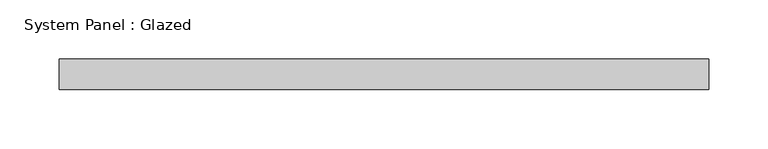
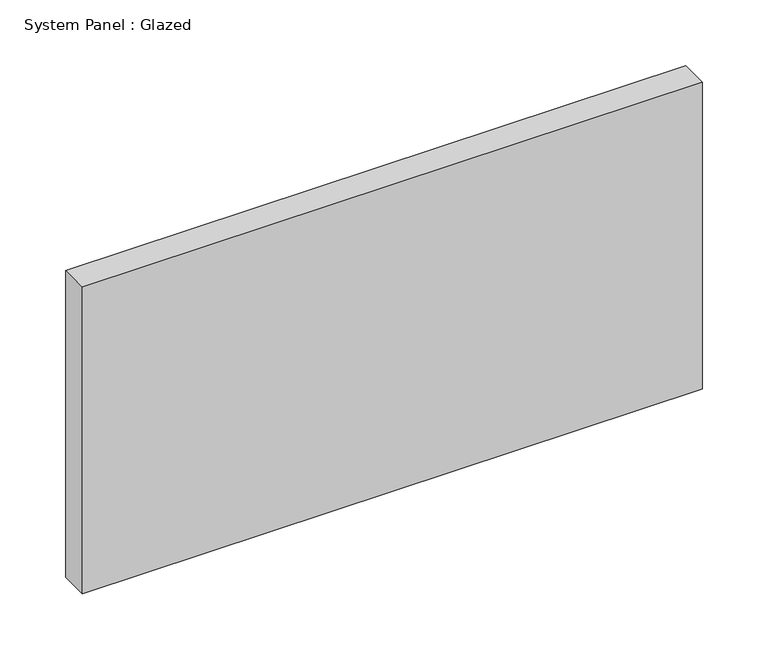
"""IFC4 building model written with IfcOpenShell, lengths in millimetres: plate geometry, System Panel : Glazed."""

from ifc_helpers import new_model, si_unit, origin, origin_with_axes, place, context, project, spatial, polyline, outline, extrude, source, transform, mapped, element, save


def system_panel_glazed_c61bacb6(model_context):
    return source(origin(), model_context, "Body", "SweptSolid", [
        extrude(outline(polyline([(273.05, 19.05), (-273.05, 19.05), (-273.05, 44.45), (273.05, 44.45), (273.05, 19.05)])), origin_with_axes(), (0.0, 0.0, 1.0), 285.75),
    ])


if __name__ == "__main__":
    model = new_model("IFC4")
    model_context = context("Model", 3, world=origin())
    ifc_project = project(units=[si_unit("LENGTHUNIT", "METRE", prefix="MILLI")], contexts=[model_context])
    site = spatial("IfcSite", under=ifc_project)
    building = spatial("IfcBuilding", under=site)
    placement = place(None, origin())
    system_panel_glazed_shape = system_panel_glazed_c61bacb6(model_context)
    element("IfcPlate", 1, ObjectType="System Panel : Glazed", at=placement, inside=building, context=model_context, shape_type="MappedRepresentation", body=[
        mapped(system_panel_glazed_shape, transform((0.0, 0.0, 0.0), x_axis=(1.0, 0.0, 0.0), y_axis=(0.0, 1.0, 0.0), z_axis=(0.0, 0.0, 1.0))),
    ])
    save(model, "model.ifc")

# Revit data of these elements
# Type "System Panel : Glazed"
#   Construction Type Id = "GSP4R"
#   Analytic Construction = "1/8 in Pilkington single glazing"
#   Visual Light Transmittance = 0.9
#   Solar Heat Gain Coefficient = 0.86
#   Heat Transfer Coefficient (U) = 1.18115 BTU/(h·ft²·°F)
#   Define Thermal Properties by = 1
# Element 1 (IfcPlate, "System Panel : Glazed")
#   Materials on its faces: "Glass"
# Materials
#   "Glass": class "Glass", colour RGB 0 128 192, transparency 0.75, Description = "Soda Lime Glass", Cost = 0
